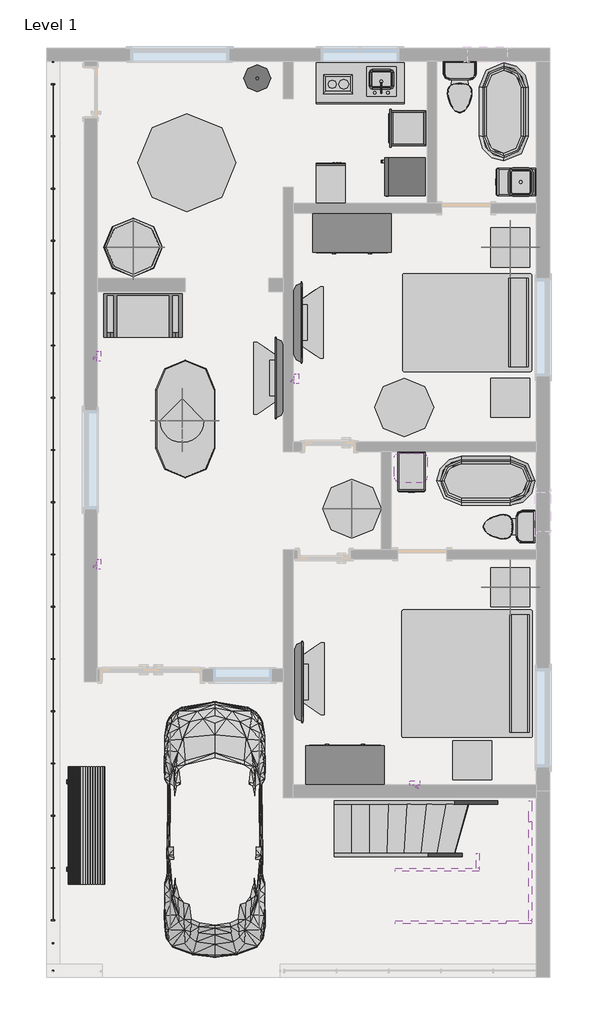
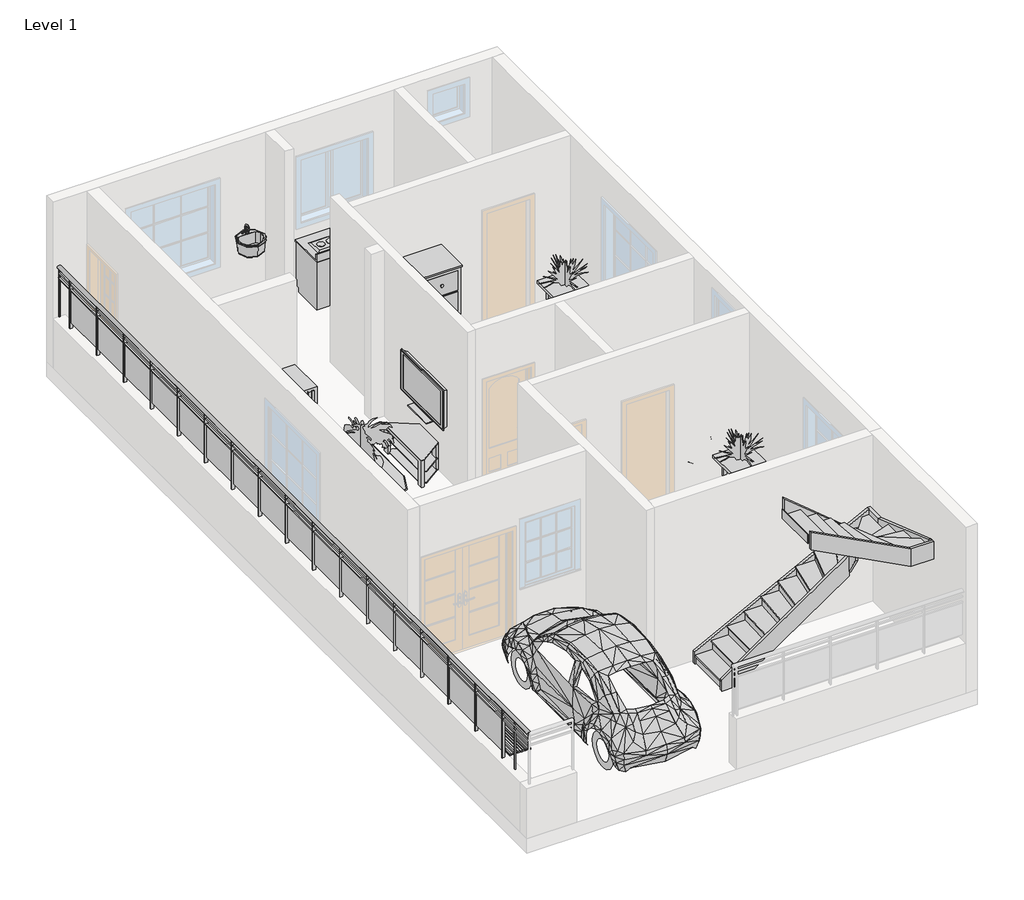
# One storey, part 2 of 2: 23 furniture elements, 10 proxies, 8 flow terminals, 8 members, 6 geographic elements, 1 railing, 1 stair flight.
"""IFC4 building model written with IfcOpenShell, lengths in millimetres."""

from ifc_helpers import new_model, si_unit, point, frame, origin, place, context, project, spatial, polyline, ellipse_curve, trimmed, outline, extrude, transform, mapped, element, save
from ifc_brep_helpers import plane_surface, extruded_surface, advanced_brep
from components import proxy_7e1014cc, proxy_fe84b772, proxy_844211aa, proxy_8b8c2dc4, rpc_beetle_rpc_beetle_3ce7ba48, rpc_picture_frame_rpc_picture_frame_c25e3fe9, proxy_c523a7b7, flow_terminal_871c2e40, flow_terminal_d49f872f, flow_terminal_62a433f7, toilet_domestic_3d_toilet_domestic_3d_f7549cf7, toilet_domestic_3d_toilet_domestic_3d_183bbd19, flow_terminal_b374fae2, furniture_39db8c53, furniture_1fc5af50, furniture_e1791683, furniture_b3f308bd, furniture_9fa109b2, furniture_c333be35, furniture_fdf74506, tv_stand_tv_stand_6ce107e5, furniture_2c34a4f9, furniture_bbcc68ce, furniture_4bee3317, furniture_5bc9ed15, furniture_c80d6d9c, geographic_element_235d1464, rpc_plant_tropical_55f6ff97, rpc_plant_tropical_agave_1_5_93a2a214, rpc_plant_tropical_japanese_fern_2_5_30b4c15b, stair_flight_d882c53c

model = new_model("IFC4")

# Units and contexts
model_context = context("Model", 3, world=origin())
ifc_project = project(units=[si_unit("LENGTHUNIT", "METRE", prefix="MILLI")], contexts=[model_context])

# Site, building, storey
site = spatial("IfcSite", under=ifc_project)
building = spatial("IfcBuilding", under=site)
storey = spatial("IfcBuildingStorey", under=building, Name="Level 1", Elevation=0.0)

# Proxies
placement = place(None, origin())
proxy_shape = proxy_7e1014cc(model_context)
element("IfcBuildingElementProxy", 1, Name="18\" x 24\" x 34 1/2\"", ObjectType="18\" x 24\" x 34 1/2\"", at=placement, inside=storey, context=model_context, shape_type="MappedRepresentation", body=[
    mapped(proxy_shape, transform((-1491.6072765, 12823.4754525, 0.0), x_axis=(-0.9999999999999998, 0.0, 0.0), y_axis=(0.0, -0.9999999999999998, 0.0), z_axis=(0.0, 0.0, 1.0))),
])
proxy_2_shape = proxy_fe84b772(model_context)
element("IfcBuildingElementProxy", 2, Name="Cook Top-2 Unit : 12\" x 18\"", ObjectType="Cook Top-2 Unit : 12\" x 18\"", at=placement, inside=storey, context=model_context, shape_type="MappedRepresentation", body=[
    mapped(proxy_2_shape, transform((-1713.6495405, 14182.6258877, 0.0), x_axis=(0.0, -1.0000000000000004, 0.0), y_axis=(1.0000000000000004, 0.0, 0.0), z_axis=(0.0, 0.0, 1.0))),
])
proxy_3_shape = proxy_844211aa(model_context)
element("IfcBuildingElementProxy", 3, Name="Kitchenette - Small : 54\"", ObjectType="Kitchenette - Small : 54\"", at=placement, inside=storey, context=model_context, shape_type="MappedRepresentation", body=[
    mapped(proxy_3_shape, transform((-1321.78704, 13801.6258877, 0.0), x_axis=(-1.0000000000000004, 0.0, 0.0), y_axis=(0.0, -1.0000000000000004, 0.0), z_axis=(0.0, 0.0, 1.0))),
])
proxy_4_shape = proxy_8b8c2dc4(model_context)
element("IfcBuildingElementProxy", 4, Name="Oven Double-Built-in : 21 1/2\" x 39 1/4\" x 21\"", ObjectType="Oven Double-Built-in : 21 1/2\" x 39 1/4\" x 21\"", at=placement, inside=storey, context=model_context, shape_type="MappedRepresentation", body=[
    mapped(proxy_4_shape, transform((-729.1156039, 13385.4509604, 0.0), x_axis=(0.0, -1.0, 0.0), y_axis=(1.0, 0.0, 0.0), z_axis=(0.0, 0.0, 1.0))),
])
rpc_beetle_rpc_beetle_shape = rpc_beetle_rpc_beetle_3ce7ba48(model_context)
element("IfcBuildingElementProxy", 5, Name="RPC Beetle : RPC Beetle", ObjectType="RPC Beetle : RPC Beetle", at=placement, inside=storey, context=model_context, shape_type="MappedRepresentation", body=[
    mapped(rpc_beetle_rpc_beetle_shape, transform((-3601.1247449, 1279.4258877, 0.0), x_axis=(1.0, 0.0, 0.0), y_axis=(0.0, 1.0, 0.0), z_axis=(0.0, 0.0, 1.0))),
])
rpc_picture_frame_rpc_picture_frame_shape = rpc_picture_frame_rpc_picture_frame_c25e3fe9(model_context)
element("IfcBuildingElementProxy", 6, Name="RPC Picture Frame : RPC Picture Frame", ObjectType="RPC Picture Frame : RPC Picture Frame", at=placement, inside=storey, context=model_context, shape_type="MappedRepresentation", body=[
    mapped(rpc_picture_frame_rpc_picture_frame_shape, transform((-489.6247449, 3209.8258877, 1828.8), x_axis=(-1.0000000000000004, 0.0, 0.0), y_axis=(0.0, -1.0000000000000004, 0.0), z_axis=(0.0, 0.0, 1.0))),
])
element("IfcBuildingElementProxy", 7, Name="RPC Picture Frame : RPC Picture Frame", ObjectType="RPC Picture Frame : RPC Picture Frame", at=placement, inside=storey, context=model_context, shape_type="MappedRepresentation", body=[
    mapped(rpc_picture_frame_rpc_picture_frame_shape, transform((-5429.9247449, 9875.6394183, 1828.8), x_axis=(0.0, 1.0, 0.0), y_axis=(-1.0, 0.0, 0.0), z_axis=(0.0, 0.0, 1.0))),
])
element("IfcBuildingElementProxy", 8, Name="RPC Picture Frame : RPC Picture Frame", ObjectType="RPC Picture Frame : RPC Picture Frame", at=placement, inside=storey, context=model_context, shape_type="MappedRepresentation", body=[
    mapped(rpc_picture_frame_rpc_picture_frame_shape, transform((-5429.9247449, 6639.0450219, 1828.8), x_axis=(0.0, 1.0, 0.0), y_axis=(-1.0, 0.0, 0.0), z_axis=(0.0, 0.0, 1.0))),
])
element("IfcBuildingElementProxy", 9, Name="RPC Picture Frame : RPC Picture Frame", ObjectType="RPC Picture Frame : RPC Picture Frame", at=placement, inside=storey, context=model_context, shape_type="MappedRepresentation", body=[
    mapped(rpc_picture_frame_rpc_picture_frame_shape, transform((-2356.5247449, 9524.6408717, 1828.8), x_axis=(0.0, 1.0, 0.0), y_axis=(-1.0, 0.0, 0.0), z_axis=(0.0, 0.0, 1.0))),
])
proxy_5_shape = proxy_c523a7b7(model_context)
element("IfcBuildingElementProxy", 10, Name="Refrigerator : 24\" x 25\" LH", ObjectType="Refrigerator : 24\" x 25\" LH", at=placement, inside=storey, context=model_context, shape_type="MappedRepresentation", body=[
    mapped(proxy_5_shape, transform((-628.1257735, 12664.9758877, 0.0), x_axis=(0.0, -1.0000000000000007, 0.0), y_axis=(1.0000000000000007, 0.0, 0.0), z_axis=(0.0, 0.0, 1.0))),
])

# Flow terminals
flow_terminal_shape = flow_terminal_871c2e40(model_context)
element("IfcFlowTerminal", 11, ObjectType="Sink Kitchen-Island : 18\" x 18\"", at=placement, inside=storey, context=model_context, shape_type="MappedRepresentation", body=[
    mapped(flow_terminal_shape, transform((-994.6355044, 14146.8712889, 0.0), x_axis=(-1.0000000000000004, 0.0, 0.0), y_axis=(0.0, -1.0000000000000004, 0.0), z_axis=(0.0, 0.0, 1.0))),
])
flow_terminal_2_shape = flow_terminal_d49f872f(model_context)
element("IfcFlowTerminal", 12, ObjectType="Sink Vanity-Round : 19\" x 19\"", at=placement, inside=storey, context=model_context, shape_type="MappedRepresentation", body=[
    mapped(flow_terminal_2_shape, transform((-3037.3764855, 14112.1068919, 609.6), x_axis=(1.0, 0.0, 0.0), y_axis=(0.0, 1.0, 0.0), z_axis=(0.0, 0.0, 1.0))),
])
flow_terminal_3_shape = flow_terminal_62a433f7(model_context)
element("IfcFlowTerminal", 13, ObjectType="Sink Vanity-Square : 20\" x 18\"", at=placement, inside=storey, context=model_context, shape_type="MappedRepresentation", body=[
    mapped(flow_terminal_3_shape, transform((-568.8139855, 8185.8804866, 914.4), x_axis=(1.0, 0.0, 0.0), y_axis=(0.0, 1.0, 0.0), z_axis=(0.0, 0.0, 1.0))),
])
element("IfcFlowTerminal", 14, ObjectType="Sink Vanity-Square : 20\" x 18\"", at=placement, inside=storey, context=model_context, shape_type="MappedRepresentation", body=[
    mapped(flow_terminal_3_shape, transform((1209.8298539, 12598.1151283, 609.6), x_axis=(0.0, -0.9999999999999999, 0.0), y_axis=(0.9999999999999999, 0.0, 0.0), z_axis=(0.0, 0.0, 1.0))),
])
toilet_domestic_3d_toilet_domestic_3d_shape = toilet_domestic_3d_toilet_domestic_3d_f7549cf7(model_context)
toilet_domestic_3d_toilet_domestic_3d_2_shape = toilet_domestic_3d_toilet_domestic_3d_183bbd19(model_context)
element("IfcFlowTerminal", 15, ObjectType="Toilet-Domestic-3D : Toilet-Domestic-3D", at=placement, inside=storey, context=model_context, shape_type="MappedRepresentation", body=[
    mapped(toilet_domestic_3d_toilet_domestic_3d_shape, transform((882.5792277, 7223.0258877, 0.0), x_axis=(0.0, -1.0000000000000004, 0.0), y_axis=(1.0000000000000004, 0.0, 0.0), z_axis=(0.0, 0.0, 1.0))),
    mapped(toilet_domestic_3d_toilet_domestic_3d_2_shape, transform((882.5792277, 7223.0258877, 0.0), x_axis=(0.0, -1.0000000000000004, 0.0), y_axis=(1.0000000000000004, 0.0, 0.0), z_axis=(0.0, 0.0, 1.0))),
])
element("IfcFlowTerminal", 16, ObjectType="Toilet-Domestic-3D : Toilet-Domestic-3D", at=placement, inside=storey, context=model_context, shape_type="MappedRepresentation", body=[
    mapped(toilet_domestic_3d_toilet_domestic_3d_shape, transform((208.8752551, 13967.3298604, 0.0), x_axis=(1.0, 0.0, 0.0), y_axis=(0.0, 1.0, 0.0), z_axis=(0.0, 0.0, 1.0))),
    mapped(toilet_domestic_3d_toilet_domestic_3d_2_shape, transform((208.8752551, 13967.3298604, 0.0), x_axis=(1.0, 0.0, 0.0), y_axis=(0.0, 1.0, 0.0), z_axis=(0.0, 0.0, 1.0))),
])
flow_terminal_4_shape = flow_terminal_b374fae2(model_context)
element("IfcFlowTerminal", 17, ObjectType="Tub-Free Standing-3D : 30\" x 60\"", at=placement, inside=storey, context=model_context, shape_type="MappedRepresentation", body=[
    mapped(flow_terminal_4_shape, transform((894.6752551, 13674.6258877, 0.0), x_axis=(1.0, 0.0, 0.0), y_axis=(0.0, 1.0, 0.0), z_axis=(0.0, 0.0, 1.0))),
])
element("IfcFlowTerminal", 18, ObjectType="Tub-Free Standing-3D : 30\" x 60\"", at=placement, inside=storey, context=model_context, shape_type="MappedRepresentation", body=[
    mapped(flow_terminal_4_shape, transform((615.2752551, 7934.2258877, 0.0), x_axis=(0.0, -1.0000000000000004, 0.0), y_axis=(1.0000000000000004, 0.0, 0.0), z_axis=(0.0, 0.0, 1.0))),
])

# Furniture
furniture_shape = furniture_39db8c53(model_context)
element("IfcFurniture", 19, ObjectType="24\"", at=placement, inside=storey, context=model_context, shape_type="MappedRepresentation", body=[
    mapped(furniture_shape, transform((-559.1624499, 8391.4258877, 0.0), x_axis=(1.0, 0.0, 0.0), y_axis=(0.0, 1.0, 0.0), z_axis=(0.0, 0.0, 1.0))),
])
element("IfcFurniture", 20, ObjectType="24\"", at=placement, inside=storey, context=model_context, shape_type="MappedRepresentation", body=[
    mapped(furniture_shape, transform((1402.6752551, 12601.1635927, 0.0), x_axis=(0.0, -0.9999999999999998, 0.0), y_axis=(0.9999999999999998, 0.0, 0.0), z_axis=(0.0, 0.0, 1.0))),
])
furniture_2_shape = furniture_1fc5af50(model_context)
element("IfcFurniture", 21, ObjectType="Bed-Standard.0001 : King 78\" x 80\"", at=placement, inside=storey, context=model_context, shape_type="MappedRepresentation", body=[
    mapped(furniture_2_shape, transform((368.770337, 5208.5144123, 0.0), x_axis=(0.0, -1.0000000000000002, 0.0), y_axis=(1.0000000000000002, 0.0, 0.0), z_axis=(0.0, 0.0, 1.0))),
])
furniture_3_shape = furniture_e1791683(model_context)
element("IfcFurniture", 22, ObjectType="Bed-Standard.0001 : Queen 60\" x 79\"", at=placement, inside=storey, context=model_context, shape_type="MappedRepresentation", body=[
    mapped(furniture_3_shape, transform((368.770337, 10669.5144123, 0.0), x_axis=(0.0, -1.0000000000000002, 0.0), y_axis=(1.0000000000000002, 0.0, 0.0), z_axis=(0.0, 0.0, 1.0))),
])
furniture_4_shape = furniture_b3f308bd(model_context)
element("IfcFurniture", 23, ObjectType="Counter Top w Sink Hole : 24\" Depth", at=placement, inside=storey, context=model_context, shape_type="MappedRepresentation", body=[
    mapped(furniture_4_shape, transform((-1855.18704, 13801.6258877, 0.0), x_axis=(-1.0000000000000004, 0.0, 0.0), y_axis=(0.0, -1.0000000000000004, 0.0), z_axis=(0.0, 0.0, 1.0))),
])
furniture_5_shape = furniture_9fa109b2(model_context)
element("IfcFurniture", 24, ObjectType="Dresser : 48\" x 72\" x 24\"", at=placement, inside=storey, context=model_context, shape_type="MappedRepresentation", body=[
    mapped(furniture_5_shape, transform((-1845.0542465, 3151.4629336, 0.0), x_axis=(-1.0000000000000004, 0.0, 0.0), y_axis=(0.0, -1.0000000000000004, 0.0), z_axis=(0.0, 0.0, 1.0))),
])
element("IfcFurniture", 25, ObjectType="Dresser : 48\" x 72\" x 24\"", at=placement, inside=storey, context=model_context, shape_type="MappedRepresentation", body=[
    mapped(furniture_5_shape, transform((-1198.3314851, 12158.1888418, 0.0), x_axis=(1.0, 0.0, 0.0), y_axis=(0.0, 1.0, 0.0), z_axis=(0.0, 0.0, 1.0))),
])
furniture_6_shape = furniture_c333be35(model_context)
element("IfcFurniture", 26, ObjectType="Entertainment Center : 72\" x 72\" x 24\"", at=placement, inside=storey, context=model_context, shape_type="MappedRepresentation", body=[
    mapped(furniture_6_shape, transform((-4718.7247449, 10950.4758877, 0.0), x_axis=(1.0, 0.0, 0.0), y_axis=(0.0, 1.0, 0.0), z_axis=(0.0, 0.0, 1.0))),
])
furniture_7_shape = furniture_fdf74506(model_context)
element("IfcFurniture", 27, ObjectType="TV - Flat Screen : 50\"", at=placement, inside=storey, context=model_context, shape_type="MappedRepresentation", body=[
    mapped(furniture_7_shape, transform((-2297.9861213, 4813.9704019, 914.4), x_axis=(0.0, 1.0000000000000002, 0.0), y_axis=(-1.0000000000000002, 0.0, 0.0), z_axis=(0.0, 0.0, 1.0))),
])
element("IfcFurniture", 28, ObjectType="TV - Flat Screen : 50\"", at=placement, inside=storey, context=model_context, shape_type="MappedRepresentation", body=[
    mapped(furniture_7_shape, transform((-2310.6861213, 10401.9704019, 914.4), x_axis=(0.0, 1.0000000000000002, 0.0), y_axis=(-1.0000000000000002, 0.0, 0.0), z_axis=(0.0, 0.0, 1.0))),
])
element("IfcFurniture", 29, ObjectType="TV - Flat Screen : 50\"", at=placement, inside=storey, context=model_context, shape_type="MappedRepresentation", body=[
    mapped(furniture_7_shape, transform((-2592.8633686, 9530.4813736, 914.4), x_axis=(0.0, -1.0000000000000004, 0.0), y_axis=(1.0000000000000004, 0.0, 0.0), z_axis=(0.0, 0.0, 1.0))),
])
tv_stand_tv_stand_shape = tv_stand_tv_stand_6ce107e5(model_context)
element("IfcFurniture", 30, ObjectType="TV Stand : TV Stand", at=placement, inside=storey, context=model_context, shape_type="MappedRepresentation", body=[
    mapped(tv_stand_tv_stand_shape, transform((-2356.5247449, 4735.6378857, 0.0), x_axis=(0.0, 1.0000000000000002, 0.0), y_axis=(-1.0000000000000002, 0.0, 0.0), z_axis=(0.0, 0.0, 1.0))),
])
element("IfcFurniture", 31, ObjectType="TV Stand : TV Stand", at=placement, inside=storey, context=model_context, shape_type="MappedRepresentation", body=[
    mapped(tv_stand_tv_stand_shape, transform((-2369.2247449, 10272.8378857, 0.0), x_axis=(0.0, 1.0000000000000002, 0.0), y_axis=(-1.0000000000000002, 0.0, 0.0), z_axis=(0.0, 0.0, 1.0))),
])
element("IfcFurniture", 32, ObjectType="TV Stand : TV Stand", at=placement, inside=storey, context=model_context, shape_type="MappedRepresentation", body=[
    mapped(tv_stand_tv_stand_shape, transform((-2534.3247449, 9659.6138898, 0.0), x_axis=(0.0, -1.0000000000000004, 0.0), y_axis=(1.0000000000000004, 0.0, 0.0), z_axis=(0.0, 0.0, 1.0))),
])
furniture_8_shape = furniture_2c34a4f9(model_context)
element("IfcFurniture", 33, ObjectType="Table-Dining Oval : 36\" x 72\"", at=placement, inside=storey, context=model_context, shape_type="MappedRepresentation", body=[
    mapped(furniture_8_shape, transform((-4416.4231056, 9301.2455599, 0.0), x_axis=(0.0, 1.0000000000000002, 0.0), y_axis=(-1.0000000000000002, 0.0, 0.0), z_axis=(0.0, 0.0, 1.0))),
])
furniture_9_shape = furniture_bbcc68ce(model_context)
element("IfcFurniture", 34, ObjectType="Table-Dining Round w Chairs : 60\" Diameter", at=placement, inside=storey, context=model_context, shape_type="MappedRepresentation", body=[
    mapped(furniture_9_shape, transform((-4136.6067122, 13072.1045763, 0.0), x_axis=(1.0, 0.0, 0.0), y_axis=(0.0, 1.0, 0.0), z_axis=(0.0, 0.0, 1.0))),
])
furniture_10_shape = furniture_4bee3317(model_context)
element("IfcFurniture", 35, ObjectType="Table-Ellipse : 60\" x 48\"", at=placement, inside=storey, context=model_context, shape_type="MappedRepresentation", body=[
    mapped(furniture_10_shape, transform((-654.7247449, 9077.2258877, 0.0), x_axis=(-1.0000000000000004, 0.0, 0.0), y_axis=(0.0, -1.0000000000000004, 0.0), z_axis=(0.0, 0.0, 1.0))),
])
element("IfcFurniture", 36, ObjectType="Table-Ellipse : 72\" x 36\"", at=placement, inside=storey, context=model_context, shape_type="MappedRepresentation", body=[
    mapped(furniture_10_shape, transform((-1467.5247449, 7502.4258877, 0.0), x_axis=(0.0, 1.0000000000000002, 0.0), y_axis=(-1.0000000000000002, 0.0, 0.0), z_axis=(0.0, 0.0, 1.0))),
])
furniture_11_shape = furniture_5bc9ed15(model_context)
element("IfcFurniture", 37, ObjectType="Table-Night Stand : 24\" x 24\" x 30\"", at=placement, inside=storey, context=model_context, shape_type="MappedRepresentation", body=[
    mapped(furniture_11_shape, transform((687.7416248, 11261.6258877, 0.0), x_axis=(1.0, 0.0, 0.0), y_axis=(0.0, 1.0, 0.0), z_axis=(0.0, 0.0, 1.0))),
])
element("IfcFurniture", 38, ObjectType="Table-Night Stand : 24\" x 24\" x 30\"", at=placement, inside=storey, context=model_context, shape_type="MappedRepresentation", body=[
    mapped(furniture_11_shape, transform((687.7416248, 8924.8258877, 0.0), x_axis=(1.0, 0.0, 0.0), y_axis=(0.0, 1.0, 0.0), z_axis=(0.0, 0.0, 1.0))),
])
element("IfcFurniture", 39, ObjectType="Table-Night Stand : 24\" x 24\" x 30\"", at=placement, inside=storey, context=model_context, shape_type="MappedRepresentation", body=[
    mapped(furniture_11_shape, transform((97.1916248, 3286.0258877, 0.0), x_axis=(1.0, 0.0, 0.0), y_axis=(0.0, 1.0, 0.0), z_axis=(0.0, 0.0, 1.0))),
])
element("IfcFurniture", 40, ObjectType="Table-Night Stand : 24\" x 24\" x 30\"", at=placement, inside=storey, context=model_context, shape_type="MappedRepresentation", body=[
    mapped(furniture_11_shape, transform((687.7416248, 5978.4258877, 0.0), x_axis=(1.0, 0.0, 0.0), y_axis=(0.0, 1.0, 0.0), z_axis=(0.0, 0.0, 1.0))),
])
furniture_12_shape = furniture_c80d6d9c(model_context)
element("IfcFurniture", 41, ObjectType="Table-Round : 36\" Diameter", at=placement, inside=storey, context=model_context, shape_type="MappedRepresentation", body=[
    mapped(furniture_12_shape, transform((-4871.1247449, 11566.4258877, 0.0), x_axis=(1.0, 0.0, 0.0), y_axis=(0.0, 1.0, 0.0), z_axis=(0.0, 0.0, 1.0))),
])

# Geographic elements
geographic_element_shape = geographic_element_235d1464(model_context)
element("IfcGeographicElement", 42, ObjectType="Park Bench : 72\"", at=placement, inside=storey, context=model_context, shape_type="MappedRepresentation", body=[
    mapped(geographic_element_shape, transform((-5633.1247449, 2574.8258877, 0.0), x_axis=(0.0, 1.0, 0.0), y_axis=(-1.0, 0.0, 0.0), z_axis=(0.0, 0.0, 1.0))),
])
rpc_plant_tropical_shape = rpc_plant_tropical_55f6ff97(model_context)
element("IfcGeographicElement", 43, ObjectType="RPC Plant - Tropical", at=placement, inside=storey, context=model_context, shape_type="MappedRepresentation", body=[
    mapped(rpc_plant_tropical_shape, transform((-4871.1247449, 11566.4258877, 762.0), x_axis=(1.0, 0.0, 0.0), y_axis=(0.0, 1.0, 0.0), z_axis=(0.0, 0.0, 1.0))),
])
rpc_plant_tropical_agave_1_5_shape = rpc_plant_tropical_agave_1_5_93a2a214(model_context)
element("IfcGeographicElement", 44, ObjectType="RPC Plant - Tropical : Agave - 1.5'", at=placement, inside=storey, context=model_context, shape_type="MappedRepresentation", body=[
    mapped(rpc_plant_tropical_agave_1_5_shape, transform((-1467.5247449, 7502.4258877, 762.0), x_axis=(1.0, 0.0, 0.0), y_axis=(0.0, 1.0, 0.0), z_axis=(0.0, 0.0, 1.0))),
])
element("IfcGeographicElement", 45, ObjectType="RPC Plant - Tropical : Agave - 1.5'", at=placement, inside=storey, context=model_context, shape_type="MappedRepresentation", body=[
    mapped(rpc_plant_tropical_agave_1_5_shape, transform((996.2752551, 6283.2258877, 762.0), x_axis=(1.0, 0.0, 0.0), y_axis=(0.0, 1.0, 0.0), z_axis=(0.0, 0.0, 1.0))),
])
element("IfcGeographicElement", 46, ObjectType="RPC Plant - Tropical : Agave - 1.5'", at=placement, inside=storey, context=model_context, shape_type="MappedRepresentation", body=[
    mapped(rpc_plant_tropical_agave_1_5_shape, transform((996.2752551, 11566.4258877, 762.0), x_axis=(1.0, 0.0, 0.0), y_axis=(0.0, 1.0, 0.0), z_axis=(0.0, 0.0, 1.0))),
])
rpc_plant_tropical_japanese_fern_2_5_shape = rpc_plant_tropical_japanese_fern_2_5_30b4c15b(model_context)
element("IfcGeographicElement", 47, ObjectType="RPC Plant - Tropical : Japanese Fern - 2.5'", at=placement, inside=storey, context=model_context, shape_type="MappedRepresentation", body=[
    mapped(rpc_plant_tropical_japanese_fern_2_5_shape, transform((-4109.1247449, 8874.0258877, 914.4), x_axis=(1.0, 0.0, 0.0), y_axis=(0.0, 1.0, 0.0), z_axis=(0.0, 0.0, 1.0))),
])

# Members
element("IfcMember", 48, ObjectType="Stringer - 2\" Width", at=placement, inside=storey, context=model_context, shape_type="SweptSolid", body=[
    extrude(outline(polyline([(229.5207224, -1746.1022736), (0.0, -1746.1022736), (0.0, -1526.2011232), (1448.1277826, 1280.536343), (1791.1058444, 1280.536343), (229.5207224, -1746.1022736)])), frame((0.0, 2909.8869757, 0.0), z_axis=(0.0, 1.0, 0.0), x_axis=(0.0, 0.0, 1.0)), (0.0, 0.0, 1.0), 50.8),
])
element("IfcMember", 49, ObjectType="Stringer - 2\" Width", at=placement, inside=storey, context=model_context, shape_type="SweptSolid", body=[
    extrude(outline(polyline([(1280.536343, 2960.6869757), (1331.336343, 2960.6869757), (1331.336343, 2635.3037531), (1280.536343, 2635.3037531), (1280.536343, 2960.6869757)])), frame((0.0, 0.0, 1448.1277826), z_axis=(0.0, 0.0, 1.0), x_axis=(1.0, 0.0, 0.0)), (0.0, 0.0, 1.0), 342.9780618),
])
element("IfcMember", 50, ObjectType="Stringer - 2\" Width", at=placement, inside=storey, context=model_context, shape_type="SweptSolid", body=[
    extrude(outline(polyline([(2635.3037531, 1791.1058444), (2635.3037531, 1448.1277826), (1096.7647998, 1978.265011), (1096.7647998, 2310.1495745), (1128.959821, 2310.1495745), (2635.3037531, 1791.1058444)])), frame((1280.536343, 0.0, 0.0), z_axis=(1.0, 0.0, 0.0), x_axis=(0.0, 1.0, 0.0)), (0.0, 0.0, 1.0), 50.8),
])
element("IfcMember", 51, ObjectType="Stringer - 2\" Width", at=placement, inside=storey, context=model_context, shape_type="SweptSolid", body=[
    extrude(outline(polyline([(1331.336343, 1096.7647998), (1331.336343, 1045.9647998), (930.0452504, 1045.9647998), (930.0452504, 1096.7647998), (1331.336343, 1096.7647998)])), frame((0.0, 0.0, 1987.7625458), z_axis=(0.0, 0.0, 1.0), x_axis=(1.0, 0.0, 0.0)), (0.0, 0.0, 1.0), 322.3870287),
])
element("IfcMember", 52, ObjectType="Stringer - 2\" Width", at=placement, inside=storey, context=model_context, shape_type="SweptSolid", body=[
    extrude(outline(polyline([(197.1288902, -1746.1022736), (0.0, -1746.1022736), (0.0, -1495.0267963), (1349.5812101, 462.8752551), (1719.7763403, 462.8752551), (197.1288902, -1746.1022736)])), frame((0.0, 2092.2258877, 0.0), z_axis=(0.0, 1.0, 0.0), x_axis=(0.0, 0.0, 1.0)), (0.0, 0.0, 1.0), 50.8),
])
element("IfcMember", 53, ObjectType="Stringer - 2\" Width", at=placement, inside=storey, context=model_context, shape_type="SweptSolid", body=[
    extrude(outline(polyline([(2143.0258877, 1935.0678912), (2143.0258877, 1384.5976326), (2126.6177625, 1384.5976326), (1914.4258877, 1725.5306428), (1914.4258877, 2264.7523132), (1937.834975, 2264.7523132), (2143.0258877, 1935.0678912)])), frame((462.8752551, 0.0, 0.0), z_axis=(1.0, 0.0, 0.0), x_axis=(0.0, 1.0, 0.0)), (0.0, 0.0, 1.0), 50.8),
])
element("IfcMember", 54, ObjectType="Stringer - 2\" Width", at=placement, inside=storey, context=model_context, shape_type="SweptSolid", body=[
    extrude(outline(polyline([(1869.9036416, 513.6752551), (2264.7523132, 513.6752551), (3344.3950183, -797.3659919), (2949.5463468, -797.3659919), (1869.9036416, 513.6752551)])), frame((0.0, 1863.6258877, 0.0), z_axis=(0.0, 1.0, 0.0), x_axis=(0.0, 0.0, 1.0)), (0.0, 0.0, 1.0), 50.8),
])
element("IfcMember", 55, ObjectType="Stringer - 2\" Width", at=placement, inside=storey, context=model_context, shape_type="SweptSolid", body=[
    extrude(outline(polyline([(1987.7625458, 930.0452504), (2310.1495745, 930.0452504), (3219.1807534, -797.3659919), (2896.7937247, -797.3659919), (1987.7625458, 930.0452504)])), frame((0.0, 1045.9647998, 0.0), z_axis=(0.0, 1.0, 0.0), x_axis=(0.0, 0.0, 1.0)), (0.0, 0.0, 1.0), 50.8),
])

# Railing
element("IfcRailing", 56, ObjectType="Glass Panel - Bottom Fill", at=placement, inside=storey, context=model_context, shape_type="SolidModel", body=[
    advanced_brep(
    [(-6077.6247449, 14462.0258877, 1828.8), (-6153.8247449, 14462.0258877, 1828.8), (-6077.6247449, 314.2258877, 1828.8), (-6153.8247449, 314.2258877, 1828.8)],
    [
        (0, 1, ellipse_curve(frame((-6115.7247449, 14462.0258877, 1828.8), z_axis=(0.0, 1.0, 0.0), x_axis=(-1.0, 0.0, 0.0)), 38.1, 28.575)),
        (1, 0, ellipse_curve(frame((-6115.7247449, 14462.0258877, 1828.8), z_axis=(0.0, 1.0, 0.0), x_axis=(-1.0, 0.0, 0.0)), 38.1, 28.575)),
        (2, 3, ellipse_curve(frame((-6115.7247449, 314.2258877, 1828.8), z_axis=(0.0, -1.0, 0.0), x_axis=(-1.0, 0.0, 0.0)), 38.1, 28.575)),
        (3, 2, ellipse_curve(frame((-6115.7247449, 314.2258877, 1828.8), z_axis=(0.0, -1.0, 0.0), x_axis=(-1.0, 0.0, 0.0)), 38.1, 28.575)),
        (0, 2),
        (3, 1),
    ],
    [
        plane_surface(frame((-6115.7247449, 14462.0258877, 1828.8), z_axis=(0.0, 1.0, 0.0), x_axis=(0.0, 0.0, -1.0))),
        plane_surface(frame((-6115.7247449, 314.2258877, 1828.8), z_axis=(0.0, -1.0, 0.0), x_axis=(0.0, 0.0, -1.0))),
        extruded_surface(trimmed(ellipse_curve(frame((-6115.7247449, 314.2258877, 1828.8), z_axis=(0.0, 1.0, 0.0), x_axis=(-1.0, 0.0, 0.0)), 38.1, 28.575), [point((-6077.6247449, 314.2258877, 1828.8))], [point((-6153.8247449, 314.2258877, 1828.8))], True, "CARTESIAN"), (0.0, 14147.8, 0.0), 14147.8),
        extruded_surface(trimmed(ellipse_curve(frame((-6115.7247449, 314.2258877, 1828.8), z_axis=(0.0, 1.0, 0.0), x_axis=(-1.0, 0.0, 0.0)), 38.1, 28.575), [point((-6153.8247449, 314.2258877, 1828.8))], [point((-6077.6247449, 314.2258877, 1828.8))], True, "CARTESIAN"), (0.0, 14147.8, 0.0), 14147.8),
    ],
    [
        (0, [[1, 2]]),
        (1, [[3, 4]]),
        (2, [[-1, 5, -4, 6]]),
        (3, [[-2, -6, -3, -5]]),
    ],
),
    extrude(outline(polyline([(-6128.4247449, 14462.0258877), (-6103.0247449, 14462.0258877), (-6103.0247449, 314.2258877), (-6128.4247449, 314.2258877), (-6128.4247449, 14462.0258877)])), frame((0.0, 0.0, 1714.5), z_axis=(0.0, 0.0, 1.0), x_axis=(1.0, 0.0, 0.0)), (0.0, 0.0, 1.0), 25.4),
    extrude(outline(polyline([(-6128.4247449, 14462.0258877), (-6103.0247449, 14462.0258877), (-6103.0247449, 314.2258877), (-6128.4247449, 314.2258877), (-6128.4247449, 14462.0258877)])), frame((0.0, 0.0, 1612.9), z_axis=(0.0, 0.0, 1.0), x_axis=(1.0, 0.0, 0.0)), (0.0, 0.0, 1.0), 25.4),
    extrude(outline(polyline([(-6141.1247449, 1107.9758877), (-6090.3247449, 1107.9758877), (-6090.3247449, 1095.2758877), (-6141.1247449, 1095.2758877), (-6141.1247449, 1107.9758877)])), frame((0.0, 0.0, 914.4), z_axis=(0.0, 0.0, 1.0), x_axis=(1.0, 0.0, 0.0)), (0.0, 0.0, 1.0), 885.6788223),
    extrude(outline(polyline([(-6109.1895879, 1914.4258877), (-6109.1895879, 1101.6258877), (-6115.5395879, 1101.6258877), (-6115.5395879, 1914.4258877), (-6109.1895879, 1914.4258877)])), frame((0.0, 0.0, 1016.0), z_axis=(0.0, 0.0, 1.0), x_axis=(1.0, 0.0, 0.0)), (0.0, 0.0, 1.0), 596.9),
    extrude(outline(polyline([(-6141.1247449, 1920.7758877), (-6090.3247449, 1920.7758877), (-6090.3247449, 1908.0758877), (-6141.1247449, 1908.0758877), (-6141.1247449, 1920.7758877)])), frame((0.0, 0.0, 914.4), z_axis=(0.0, 0.0, 1.0), x_axis=(1.0, 0.0, 0.0)), (0.0, 0.0, 1.0), 885.6788223),
    extrude(outline(polyline([(-6109.1895879, 2727.2258877), (-6109.1895879, 1914.4258877), (-6115.5395879, 1914.4258877), (-6115.5395879, 2727.2258877), (-6109.1895879, 2727.2258877)])), frame((0.0, 0.0, 1016.0), z_axis=(0.0, 0.0, 1.0), x_axis=(1.0, 0.0, 0.0)), (0.0, 0.0, 1.0), 596.9),
    extrude(outline(polyline([(-6141.1247449, 2733.5758877), (-6090.3247449, 2733.5758877), (-6090.3247449, 2720.8758877), (-6141.1247449, 2720.8758877), (-6141.1247449, 2733.5758877)])), frame((0.0, 0.0, 914.4), z_axis=(0.0, 0.0, 1.0), x_axis=(1.0, 0.0, 0.0)), (0.0, 0.0, 1.0), 885.6788223),
    extrude(outline(polyline([(-6109.1895879, 3540.0258877), (-6109.1895879, 2727.2258877), (-6115.5395879, 2727.2258877), (-6115.5395879, 3540.0258877), (-6109.1895879, 3540.0258877)])), frame((0.0, 0.0, 1016.0), z_axis=(0.0, 0.0, 1.0), x_axis=(1.0, 0.0, 0.0)), (0.0, 0.0, 1.0), 596.9),
    extrude(outline(polyline([(-6141.1247449, 3546.3758877), (-6090.3247449, 3546.3758877), (-6090.3247449, 3533.6758877), (-6141.1247449, 3533.6758877), (-6141.1247449, 3546.3758877)])), frame((0.0, 0.0, 914.4), z_axis=(0.0, 0.0, 1.0), x_axis=(1.0, 0.0, 0.0)), (0.0, 0.0, 1.0), 885.6788223),
    extrude(outline(polyline([(-6109.1895879, 4352.8258877), (-6109.1895879, 3540.0258877), (-6115.5395879, 3540.0258877), (-6115.5395879, 4352.8258877), (-6109.1895879, 4352.8258877)])), frame((0.0, 0.0, 1016.0), z_axis=(0.0, 0.0, 1.0), x_axis=(1.0, 0.0, 0.0)), (0.0, 0.0, 1.0), 596.9),
    extrude(outline(polyline([(-6141.1247449, 4359.1758877), (-6090.3247449, 4359.1758877), (-6090.3247449, 4346.4758877), (-6141.1247449, 4346.4758877), (-6141.1247449, 4359.1758877)])), frame((0.0, 0.0, 914.4), z_axis=(0.0, 0.0, 1.0), x_axis=(1.0, 0.0, 0.0)), (0.0, 0.0, 1.0), 885.6788223),
    extrude(outline(polyline([(-6109.1895879, 5165.6258877), (-6109.1895879, 4352.8258877), (-6115.5395879, 4352.8258877), (-6115.5395879, 5165.6258877), (-6109.1895879, 5165.6258877)])), frame((0.0, 0.0, 1016.0), z_axis=(0.0, 0.0, 1.0), x_axis=(1.0, 0.0, 0.0)), (0.0, 0.0, 1.0), 596.9),
    extrude(outline(polyline([(-6141.1247449, 5171.9758877), (-6090.3247449, 5171.9758877), (-6090.3247449, 5159.2758877), (-6141.1247449, 5159.2758877), (-6141.1247449, 5171.9758877)])), frame((0.0, 0.0, 914.4), z_axis=(0.0, 0.0, 1.0), x_axis=(1.0, 0.0, 0.0)), (0.0, 0.0, 1.0), 885.6788223),
    extrude(outline(polyline([(-6109.1895879, 5978.4258877), (-6109.1895879, 5165.6258877), (-6115.5395879, 5165.6258877), (-6115.5395879, 5978.4258877), (-6109.1895879, 5978.4258877)])), frame((0.0, 0.0, 1016.0), z_axis=(0.0, 0.0, 1.0), x_axis=(1.0, 0.0, 0.0)), (0.0, 0.0, 1.0), 596.9),
    extrude(outline(polyline([(-6141.1247449, 5984.7758877), (-6090.3247449, 5984.7758877), (-6090.3247449, 5972.0758877), (-6141.1247449, 5972.0758877), (-6141.1247449, 5984.7758877)])), frame((0.0, 0.0, 914.4), z_axis=(0.0, 0.0, 1.0), x_axis=(1.0, 0.0, 0.0)), (0.0, 0.0, 1.0), 885.6788223),
    extrude(outline(polyline([(-6109.1895879, 6791.2258877), (-6109.1895879, 5978.4258877), (-6115.5395879, 5978.4258877), (-6115.5395879, 6791.2258877), (-6109.1895879, 6791.2258877)])), frame((0.0, 0.0, 1016.0), z_axis=(0.0, 0.0, 1.0), x_axis=(1.0, 0.0, 0.0)), (0.0, 0.0, 1.0), 596.9),
    extrude(outline(polyline([(-6141.1247449, 6797.5758877), (-6090.3247449, 6797.5758877), (-6090.3247449, 6784.8758877), (-6141.1247449, 6784.8758877), (-6141.1247449, 6797.5758877)])), frame((0.0, 0.0, 914.4), z_axis=(0.0, 0.0, 1.0), x_axis=(1.0, 0.0, 0.0)), (0.0, 0.0, 1.0), 885.6788223),
    extrude(outline(polyline([(-6109.1895879, 7604.0258877), (-6109.1895879, 6791.2258877), (-6115.5395879, 6791.2258877), (-6115.5395879, 7604.0258877), (-6109.1895879, 7604.0258877)])), frame((0.0, 0.0, 1016.0), z_axis=(0.0, 0.0, 1.0), x_axis=(1.0, 0.0, 0.0)), (0.0, 0.0, 1.0), 596.9),
    extrude(outline(polyline([(-6141.1247449, 7610.3758877), (-6090.3247449, 7610.3758877), (-6090.3247449, 7597.6758877), (-6141.1247449, 7597.6758877), (-6141.1247449, 7610.3758877)])), frame((0.0, 0.0, 914.4), z_axis=(0.0, 0.0, 1.0), x_axis=(1.0, 0.0, 0.0)), (0.0, 0.0, 1.0), 885.6788223),
    extrude(outline(polyline([(-6109.1895879, 8416.8258877), (-6109.1895879, 7604.0258877), (-6115.5395879, 7604.0258877), (-6115.5395879, 8416.8258877), (-6109.1895879, 8416.8258877)])), frame((0.0, 0.0, 1016.0), z_axis=(0.0, 0.0, 1.0), x_axis=(1.0, 0.0, 0.0)), (0.0, 0.0, 1.0), 596.9),
    extrude(outline(polyline([(-6141.1247449, 8423.1758877), (-6090.3247449, 8423.1758877), (-6090.3247449, 8410.4758877), (-6141.1247449, 8410.4758877), (-6141.1247449, 8423.1758877)])), frame((0.0, 0.0, 914.4), z_axis=(0.0, 0.0, 1.0), x_axis=(1.0, 0.0, 0.0)), (0.0, 0.0, 1.0), 885.6788223),
    extrude(outline(polyline([(-6109.1895879, 9229.6258877), (-6109.1895879, 8416.8258877), (-6115.5395879, 8416.8258877), (-6115.5395879, 9229.6258877), (-6109.1895879, 9229.6258877)])), frame((0.0, 0.0, 1016.0), z_axis=(0.0, 0.0, 1.0), x_axis=(1.0, 0.0, 0.0)), (0.0, 0.0, 1.0), 596.9),
    extrude(outline(polyline([(-6141.1247449, 9235.9758877), (-6090.3247449, 9235.9758877), (-6090.3247449, 9223.2758877), (-6141.1247449, 9223.2758877), (-6141.1247449, 9235.9758877)])), frame((0.0, 0.0, 914.4), z_axis=(0.0, 0.0, 1.0), x_axis=(1.0, 0.0, 0.0)), (0.0, 0.0, 1.0), 885.6788223),
    extrude(outline(polyline([(-6109.1895879, 10042.4258877), (-6109.1895879, 9229.6258877), (-6115.5395879, 9229.6258877), (-6115.5395879, 10042.4258877), (-6109.1895879, 10042.4258877)])), frame((0.0, 0.0, 1016.0), z_axis=(0.0, 0.0, 1.0), x_axis=(1.0, 0.0, 0.0)), (0.0, 0.0, 1.0), 596.9),
    extrude(outline(polyline([(-6141.1247449, 10048.7758877), (-6090.3247449, 10048.7758877), (-6090.3247449, 10036.0758877), (-6141.1247449, 10036.0758877), (-6141.1247449, 10048.7758877)])), frame((0.0, 0.0, 914.4), z_axis=(0.0, 0.0, 1.0), x_axis=(1.0, 0.0, 0.0)), (0.0, 0.0, 1.0), 885.6788223),
    extrude(outline(polyline([(-6109.1895879, 10855.2258877), (-6109.1895879, 10042.4258877), (-6115.5395879, 10042.4258877), (-6115.5395879, 10855.2258877), (-6109.1895879, 10855.2258877)])), frame((0.0, 0.0, 1016.0), z_axis=(0.0, 0.0, 1.0), x_axis=(1.0, 0.0, 0.0)), (0.0, 0.0, 1.0), 596.9),
    extrude(outline(polyline([(-6141.1247449, 10861.5758877), (-6090.3247449, 10861.5758877), (-6090.3247449, 10848.8758877), (-6141.1247449, 10848.8758877), (-6141.1247449, 10861.5758877)])), frame((0.0, 0.0, 914.4), z_axis=(0.0, 0.0, 1.0), x_axis=(1.0, 0.0, 0.0)), (0.0, 0.0, 1.0), 885.6788223),
    extrude(outline(polyline([(-6109.1895879, 11668.0258877), (-6109.1895879, 10855.2258877), (-6115.5395879, 10855.2258877), (-6115.5395879, 11668.0258877), (-6109.1895879, 11668.0258877)])), frame((0.0, 0.0, 1016.0), z_axis=(0.0, 0.0, 1.0), x_axis=(1.0, 0.0, 0.0)), (0.0, 0.0, 1.0), 596.9),
    extrude(outline(polyline([(-6141.1247449, 11674.3758877), (-6090.3247449, 11674.3758877), (-6090.3247449, 11661.6758877), (-6141.1247449, 11661.6758877), (-6141.1247449, 11674.3758877)])), frame((0.0, 0.0, 914.4), z_axis=(0.0, 0.0, 1.0), x_axis=(1.0, 0.0, 0.0)), (0.0, 0.0, 1.0), 885.6788223),
    extrude(outline(polyline([(-6109.1895879, 12480.8258877), (-6109.1895879, 11668.0258877), (-6115.5395879, 11668.0258877), (-6115.5395879, 12480.8258877), (-6109.1895879, 12480.8258877)])), frame((0.0, 0.0, 1016.0), z_axis=(0.0, 0.0, 1.0), x_axis=(1.0, 0.0, 0.0)), (0.0, 0.0, 1.0), 596.9),
    extrude(outline(polyline([(-6141.1247449, 12487.1758877), (-6090.3247449, 12487.1758877), (-6090.3247449, 12474.4758877), (-6141.1247449, 12474.4758877), (-6141.1247449, 12487.1758877)])), frame((0.0, 0.0, 914.4), z_axis=(0.0, 0.0, 1.0), x_axis=(1.0, 0.0, 0.0)), (0.0, 0.0, 1.0), 885.6788223),
    extrude(outline(polyline([(-6109.1895879, 13293.6258877), (-6109.1895879, 12480.8258877), (-6115.5395879, 12480.8258877), (-6115.5395879, 13293.6258877), (-6109.1895879, 13293.6258877)])), frame((0.0, 0.0, 1016.0), z_axis=(0.0, 0.0, 1.0), x_axis=(1.0, 0.0, 0.0)), (0.0, 0.0, 1.0), 596.9),
    extrude(outline(polyline([(-6141.1247449, 13299.9758877), (-6090.3247449, 13299.9758877), (-6090.3247449, 13287.2758877), (-6141.1247449, 13287.2758877), (-6141.1247449, 13299.9758877)])), frame((0.0, 0.0, 914.4), z_axis=(0.0, 0.0, 1.0), x_axis=(1.0, 0.0, 0.0)), (0.0, 0.0, 1.0), 885.6788223),
    extrude(outline(polyline([(-6109.1895879, 14106.4258877), (-6109.1895879, 13293.6258877), (-6115.5395879, 13293.6258877), (-6115.5395879, 14106.4258877), (-6109.1895879, 14106.4258877)])), frame((0.0, 0.0, 1016.0), z_axis=(0.0, 0.0, 1.0), x_axis=(1.0, 0.0, 0.0)), (0.0, 0.0, 1.0), 596.9),
    extrude(outline(polyline([(-6141.1247449, 14112.7758877), (-6090.3247449, 14112.7758877), (-6090.3247449, 14100.0758877), (-6141.1247449, 14100.0758877), (-6141.1247449, 14112.7758877)])), frame((0.0, 0.0, 914.4), z_axis=(0.0, 0.0, 1.0), x_axis=(1.0, 0.0, 0.0)), (0.0, 0.0, 1.0), 885.6788223),
    extrude(outline(polyline([(-6125.2497449, 755.5508877), (-6106.1997449, 755.5508877), (-6106.1997449, 736.5008877), (-6125.2497449, 736.5008877), (-6125.2497449, 755.5508877)])), frame((0.0, 0.0, 914.4), z_axis=(0.0, 0.0, 1.0), x_axis=(1.0, 0.0, 0.0)), (0.0, 0.0, 1.0), 885.6788223),
    extrude(outline(polyline([(-6125.2497449, 326.9258877), (-6106.1997449, 326.9258877), (-6106.1997449, 307.8758877), (-6125.2497449, 307.8758877), (-6125.2497449, 326.9258877)])), frame((0.0, 0.0, 914.4), z_axis=(0.0, 0.0, 1.0), x_axis=(1.0, 0.0, 0.0)), (0.0, 0.0, 1.0), 885.6788223),
    extrude(outline(polyline([(-6125.2497449, 14468.3758877), (-6106.1997449, 14468.3758877), (-6106.1997449, 14449.3258877), (-6125.2497449, 14449.3258877), (-6125.2497449, 14468.3758877)])), frame((0.0, 0.0, 914.4), z_axis=(0.0, 0.0, 1.0), x_axis=(1.0, 0.0, 0.0)), (0.0, 0.0, 1.0), 885.6788223),
])

# Stair flight
stair_flight_shape = stair_flight_d882c53c(model_context)
element("IfcStairFlight", 57, ObjectType="2\" Tread 1\" Nosing 1/4\" Riser", at=placement, inside=storey, context=model_context, shape_type="MappedRepresentation", body=[
    mapped(stair_flight_shape, transform((0.0, 0.0, 0.0), x_axis=(1.0, 0.0, 0.0), y_axis=(0.0, 1.0, 0.0), z_axis=(0.0, 0.0, 1.0))),
])

save(model, "model.ifc")

# Revit data of these elements
# Type "18\" x 24\" x 34 1/2\""
#   Label = "T"
#   Assembly Code = "E1090400"
#   Depth = 2' - 0"
#   Height = 2' - 10 1/2"
#   Width = 1' - 6"
#   Panel Face Material = Plastic, Opaque Black
#   Trach Compact. Material = Steel, Paint Finish, Ivory, Matte
#   Default Elevation = 0
# Type "Cook Top-2 Unit : 12\" x 18\""
#   Assembly Code = "E1090400"
#   Counter Height = 3' - 0"
#   Depth = 1' - 6"
#   Width = 1' - 0"
#   Burner Material = Steel, Chrome Plated
#   Cooktop Material = Steel, Polished
#   Default Elevation = 0
# Type "Kitchenette - Small : 54\""
#   Assembly Code = "E1090400"
#   Width = 4' - 6"
#   Height = 2' - 10 1/2"
#   Depth = 2' - 0"
#   Toe Depth = 0' - 3"
#   Toe Height = 0' - 3 1/2"
#   Cabinet Material = Cabinets
#   Door/Drawer Material = Cabinets
#   Handle Material = Cabinets - Handles
#   Default Elevation = 0
# Type "Oven Double-Built-in : 21 1/2\" x 39 1/4\" x 21\""
#   Label = "OVEN"
#   Assembly Code = "E1090400"
#   Depth = 1' - 9"
#   Height = 3' - 3 1/4"
#   Width = 1' - 9 1/2"
#   Oven Material = Metal - Stainless Steel, Polished
#   Default Elevation = 0
# Type "RPC Beetle : RPC Beetle"
#   built-in parameter 1005195 = "RPC-16-0U6E-L4EG-ENH1-J3KF-SVEL-0TX4-C0"
#   Height = 0
# Type "RPC Picture Frame : RPC Picture Frame"
#   built-in parameter 1005198 = "{2, 15},{39, RPC-16-8M5E-0H3T-F0AH-3U0K-JLQ7-G28B-AU},{1, 0},{1, 0},{2, 19},{1, 8},{5, Color},{1, 0},{1, 0},{3, 0.8},{3, 0.8},{3, 0.8},{1, 8},{7, BBoxMin},{1, 0},{1, 0},{1, 0},{1, 0},{1, 0},{1, 8},{7, BBoxMax},{1, 0},{1, 0},{1, 0},{1, 0},{1, 0},{2, 11},{9, RPCTypeId},{1, 0},{1, 0},{39, RPC-16-8M5E-0H3T-F0AH-3U0K-JLQ7-G28B-AU},{1, 6},{14, RPCPlantHeight},{1, 0},{1, 0},{5, 0.625},{2, 11},{7, keyword},{1, 0},{1, 0},{33, :RPCs:Office Clutter:Geometry:RPC},{2, 11},{8, category},{1, 0},{1, 0},{14, Office Clutter},{2, 11},{12, LocalizedUID},{1, 0},{1, 0},{13, Picture Frame},{2, 14},{6, Height},{1, 0},{1, 0},{5, 0.625},{1, 2},{16, Cast Reflections},{1, 0},{1, 0},{1, 0},{1, 2},{8, Portrait},{1, 0},{1, 0},{1, 1},{1, 2},{5, Stand},{1, 0},{1, 0},{1, 1},{2, 11},{10, RPCL_Frame},{1, 0},{1, 0},{5, Frame},{1, 4},{14, Frame Material},{1, 0},{1, 0},{1, 0},{2, 11},{12, RPCL_Picture},{1, 0},{1, 0},{7, Picture},{2, 11},{15, Picture Preview},{1, 0},{1, 0},{65, __RPC:/object data/textures/object/Photo/Photo0/textures/Portrait},{2, 11},{17, i_Picture Preview},{1, 0},{1, 0},{0, },{1, 2},{18, Use Custom Picture},{1, 0},{1, 0},{1, 0},{2, 11},{17, Picture File Name},{1, 0},{1, 0},{0, },{21, assetlibrary_base.fbx},{1, 5},"
#   built-in parameter 1005195 = "RPC-16-8M5E-0H3T-F0AH-3U0K-JLQ7-G28B-AU"
#   Height = 0
# Type "Refrigerator : 24\" x 25\" LH"
#   Label = "REF."
#   Assembly Code = "E1090400"
#   Depth = 2' - 0 3/4"
#   Handle = 0' - 1 1/2"
#   Height = 5' - 3 1/2"
#   Rear Clearance = 0' - 2"
#   Top Door Height = 1' - 8"
#   Width = 1' - 11 1/2"
#   Material = Steel, Paint Finish, Ivory, Glossy
#   Default Elevation = 0
# Type "Sink Kitchen-Island : 18\" x 18\""
#   Assembly Code = "D2010410"
#   Counter Height = 3' - 0"
#   Depth = 1' - 6"
#   Width = 1' - 6"
#   Faucet Material = Steel, Polished
#   Sink Material = Steel, Polished
#   Default Elevation = 0
# Type "Sink Vanity-Round : 19\" x 19\""
#   Assembly Code = "D2010400"
#   Top Of Counter = 2' - 7"
#   Basin Material = Porcelain, Linen
#   Faucet Material = Steel, Polished
#   Default Elevation = 0
# Type "Sink Vanity-Square : 20\" x 18\""
#   Assembly Code = "D2010400"
#   Counter Height = 2' - 7"
#   Depth = 1' - 6"
#   Width = 1' - 8"
#   Basin Material = Porcelain, Linen
#   Faucet Material = Steel, Polished
#   Default Elevation = 0
# Type "Toilet-Domestic-3D : Toilet-Domestic-3D"
#   Assembly Code = "D2010110"
#   Toilet - Bowl/Basin Material = Porcelain, Linen
#   Toilet - Seat Material = Laminate, Linen, Matte
#   Default Elevation = 0
# Type "Tub-Free Standing-3D : 30\" x 60\""
#   Assembly Code = "D2010110"
#   Height = 1' - 6"
#   Length = 5' - 0"
#   Width = 2' - 6"
#   Tub Material = Porcelain, Ivory
#   Default Elevation = 0
# Type "24\""
#   Assembly Code = "C1030410"
#   Depth = 2' - 0"
#   Height = 2' - 5 1/2"
#   Toe Depth = 0' - 3"
#   Toe Height = 0' - 3 1/2"
#   Width = 1' - 5"
#   Cabinet Material = none
#   Door/Drawer Material = none
#   Handle Material = Cabinets - Handles
#   Default Elevation = 0
# Type "Bed-Standard.0001 : King 78\" x 80\""
#   Assembly Code = "E2020200"
#   Length = 6' - 8"
#   Width = 6' - 6"
#   Leg Material = Steel, Chrome Plated
#   Mattress Material = Linen, Beige
#   Default Elevation = 0
# Type "Bed-Standard.0001 : Queen 60\" x 79\""
#   Assembly Code = "E2020200"
#   Length = 6' - 7"
#   Width = 5' - 0"
#   Leg Material = Steel, Chrome Plated
#   Mattress Material = Linen, White
#   Default Elevation = 0
# Type "Counter Top w Sink Hole : 24\" Depth"
#   Assembly Code = "C1030400"
#   Counter Thickness = 0' - 1 1/2"
#   Depth = 2' - 1"
#   Height = 3' - 0"
#   Length [instance default] = 8' - 0"
#   Sink Location [instance default] = 2' - 0"
#   Sink Location To Wall [instance default] = 0' - 6"
#   Sink Opening Depth [instance default] = 1' - 3"
#   Sink Opening Width [instance default] = 2' - 3"
#   Counter Top Material = none
#   Default Elevation = 0
# Type "Dresser : 48\" x 72\" x 24\""
#   Assembly Code = "E2020200"
#   Depth = 2' - 0"
#   Height = 6' - 0"
#   Width = 4' - 0"
#   Dresser Material = Laminate - Ivory, Glossy
#   Drawer Material = Laminate, Ivory, Matte
#   Knob Material = Cherry
#   Default Elevation = 0
# Type "Entertainment Center : 72\" x 72\" x 24\""
#   Assembly Code = "E2020200"
#   Center Width = 2' - 8"
#   Depth = 2' - 0"
#   Height = 5' - 0"
#   Width = 4' - 0"
#   Material = none
#   Default Elevation = 0
# Type "TV - Flat Screen : 50\""
#   SinAng = 0' - 0.0193"
#   L = 3' - 7.57782"
#   H = 2' - 0.51477"
#   Thickness = 0' - 4.33071"
#   Diagonal = 4' - 2"
#   CosAng = 0' - 0.03431"
#   Stand [instance default] = yes
#   Default Elevation = 0
# Type "TV Stand : TV Stand"
#   Depth = 1' - 6"
#   Width = 3' - 8"
#   Height = 1' - 7 1/2"
#   Finish = Melamine - Gray
#   Default Elevation = 0
# Type "Table-Dining Oval : 36\" x 72\""
#   Assembly Code = "E2020200"
#   Length = 6' - 0"
#   Width = 3' - 0"
#   Base Material = Steel, Chrome Plated
#   Top Material = Glass - Clear, Grey
#   Default Elevation = 0
#   Description = (empty or 0)
# Type "Table-Dining Round w Chairs : 60\" Diameter"
#   Assembly Code = "E2020200"
#   Radius = 2' - 6"
#   Diameter = 5' - 0"
#   Height = 2' - 6"
#   Chairs = 6
#   Base Material = Pine
#   Top Material = Laminate, Linen, Matte
#   Default Elevation = 0
# Type "Table-Ellipse : 60\" x 48\""
#   Assembly Code = "E2020200"
#   Half Width = 1' - 6"
#   Half Length = 1' - 6"
#   Height = 2' - 6"
#   Length = 3' - 0"
#   Width = 3' - 0"
#   Base Material = Birch
#   Top Material = Birch
#   Default Elevation = 0
# Type "Table-Ellipse : 72\" x 36\""
#   Assembly Code = "E2020200"
#   Half Width = 1' - 6"
#   Half Length = 1' - 6"
#   Height = 2' - 6"
#   Length = 3' - 0"
#   Width = 3' - 0"
#   Base Material = Birch
#   Top Material = Laminate - Black
#   Default Elevation = 0
# Type "Table-Night Stand : 24\" x 24\" x 30\""
#   Assembly Code = "E2020200"
#   Depth = 2' - 0"
#   Height = 2' - 6"
#   Width = 2' - 0"
#   Base Material = Birch
#   Top Material = Laminate, Ivory, Matte
#   Default Elevation = 0
# Type "Table-Round : 36\" Diameter"
#   Assembly Code = "E2020200"
#   Base Radius = 0' - 10"
#   Height = 2' - 6"
#   Radius = 1' - 6"
#   Base Material = Steel, Chrome Plated
#   Top Material = Birch
#   Default Elevation = 0
# Type "Park Bench : 72\""
#   Length = 6' - 0"
#   Seat Material = Wood - Teak
#   Frame Material = Steel, Paint Finish, Dark Gray, Matte
# Type "RPC Plant - Tropical"
#   built-in parameter 1005198 = "{2, 15},{39, RPC-16-FWM5-GM7X-C67P-4000-ST1L-LVER-AU},{1, 0},{1, 0},{2, 13},{1, 8},{5, Color},{1, 0},{1, 0},{3, 0.8},{3, 0.8},{3, 0.8},{1, 8},{7, BBoxMin},{1, 0},{1, 0},{1, 0},{1, 0},{1, 0},{1, 8},{7, BBoxMax},{1, 0},{1, 0},{1, 0},{1, 0},{1, 0},{2, 11},{9, RPCTypeId},{1, 0},{1, 0},{39, RPC-16-FWM5-GM7X-C67P-4000-ST1L-LVER-AU},{1, 6},{14, RPCPlantHeight},{1, 0},{1, 0},{1, 3},{2, 11},{7, keyword},{1, 0},{1, 0},{35, :RPCs:Shrubs [General]:Geometry:RPC},{2, 11},{8, category},{1, 0},{1, 0},{16, Shrubs [General]},{2, 11},{12, LocalizedUID},{1, 0},{1, 0},{10, Crane Lily},{2, 14},{6, Height},{1, 0},{1, 0},{1, 3},{1, 2},{16, Cast Reflections},{1, 0},{1, 0},{1, 0},{1, 2},{12, Cast Shadows},{1, 0},{1, 0},{1, 1},{1, 2},{9, Lock View},{1, 0},{1, 0},{1, 0},{1, 4},{5, ViewC},{1, 0},{1, 0},{1, 0},{21, assetlibrary_base.fbx},{1, 5},"
#   built-in parameter 1005195 = "RPC-16-FWM5-GM7X-C67P-4000-ST1L-LVER-AU"
#   Assembly Code = "G2050500"
#   Height = 3' - 0"
#   Default Elevation = 0
# Type "RPC Plant - Tropical : Agave - 1.5'"
#   built-in parameter 1005198 = "{2, 15},{39, RPC-16-G1GJ-63FX-7K5P-N000-ST1L-LVER-AU},{1, 0},{1, 0},{2, 13},{1, 8},{5, Color},{1, 0},{1, 0},{3, 0.8},{3, 0.8},{3, 0.8},{1, 8},{7, BBoxMin},{1, 0},{1, 0},{1, 0},{1, 0},{1, 0},{1, 8},{7, BBoxMax},{1, 0},{1, 0},{1, 0},{1, 0},{1, 0},{2, 11},{9, RPCTypeId},{1, 0},{1, 0},{39, RPC-16-G1GJ-63FX-7K5P-N000-ST1L-LVER-AU},{1, 6},{14, RPCPlantHeight},{1, 0},{1, 0},{3, 1.5},{2, 11},{7, keyword},{1, 0},{1, 0},{35, :RPCs:Plants [General]:Geometry:RPC},{2, 11},{8, category},{1, 0},{1, 0},{16, Plants [General]},{2, 11},{12, LocalizedUID},{1, 0},{1, 0},{5, Agave},{2, 14},{6, Height},{1, 0},{1, 0},{3, 1.5},{1, 2},{16, Cast Reflections},{1, 0},{1, 0},{1, 0},{1, 2},{12, Cast Shadows},{1, 0},{1, 0},{1, 1},{1, 2},{9, Lock View},{1, 0},{1, 0},{1, 0},{1, 4},{5, ViewC},{1, 0},{1, 0},{1, 0},{21, assetlibrary_base.fbx},{1, 5},"
#   built-in parameter 1005195 = "RPC-16-G1GJ-63FX-7K5P-N000-ST1L-LVER-AU"
#   Type Comments = "Agave"
#   Assembly Code = "G2050500"
#   Height = 1' - 6"
#   Default Elevation = 0
# Type "RPC Plant - Tropical : Japanese Fern - 2.5'"
#   built-in parameter 1005198 = "{2, 15},{39, RPC-16-G1GK-JAPX-7J4P-Q000-ST1L-LVER-AU},{1, 0},{1, 0},{2, 13},{1, 8},{5, Color},{1, 0},{1, 0},{3, 0.8},{3, 0.8},{3, 0.8},{1, 8},{7, BBoxMin},{1, 0},{1, 0},{1, 0},{1, 0},{1, 0},{1, 8},{7, BBoxMax},{1, 0},{1, 0},{1, 0},{1, 0},{1, 0},{2, 11},{9, RPCTypeId},{1, 0},{1, 0},{39, RPC-16-G1GK-JAPX-7J4P-Q000-ST1L-LVER-AU},{1, 6},{14, RPCPlantHeight},{1, 0},{1, 0},{3, 2.5},{2, 11},{7, keyword},{1, 0},{1, 0},{35, :RPCs:Shrubs [General]:Geometry:RPC},{2, 11},{8, category},{1, 0},{1, 0},{16, Shrubs [General]},{2, 11},{12, LocalizedUID},{1, 0},{1, 0},{13, Japanese Fern},{2, 14},{6, Height},{1, 0},{1, 0},{3, 2.5},{1, 2},{16, Cast Reflections},{1, 0},{1, 0},{1, 0},{1, 2},{12, Cast Shadows},{1, 0},{1, 0},{1, 1},{1, 2},{9, Lock View},{1, 0},{1, 0},{1, 0},{1, 4},{5, ViewC},{1, 0},{1, 0},{1, 0},{21, assetlibrary_base.fbx},{1, 5},"
#   built-in parameter 1005195 = "RPC-16-G1GK-JAPX-7J4P-Q000-ST1L-LVER-AU"
#   Type Comments = "Japanese Fern"
#   Assembly Code = "G2050500"
#   Height = 2' - 6"
#   Default Elevation = 0
# Type "Glass Panel - Bottom Fill"
#   Assembly Code = "C2010400"
#   built-in parameter 1008612 = 0.0416667 (stored number, unit not read)
#   built-in parameter 1008611 = 0.0416667 (stored number, unit not read)
#   built-in parameter 1008609 = 0.333333 (stored number, unit not read)
#   built-in parameter 1008604 = 0.166667 (stored number, unit not read)
#   built-in parameter 1008603 = 0.166667 (stored number, unit not read)
#   Railing Height = 3' - 0"
#   built-in parameter 1008630 = 2
#   built-in parameter 1008610 = 2
#   built-in parameter 1008618 = Baluster - Square : 3/4"
# Element 1 (IfcBuildingElementProxy, "18\" x 24\" x 34 1/2\"")
#   Phase Created = New Construction
#   Materials on its faces: "Steel, Paint Finish, Ivory, Matte", "Plastic, Opaque Black"
# Element 2 (IfcBuildingElementProxy, "Cook Top-2 Unit : 12\" x 18\"")
#   Phase Created = New Construction
#   Materials on its faces: "Steel, Chrome Plated", "Steel, Polished"
# Element 3 (IfcBuildingElementProxy, "Kitchenette - Small : 54\"")
#   Phase Created = New Construction
#   Materials on its faces: "Cabinets", "Cabinets - Handles"
# Element 4 (IfcBuildingElementProxy, "Oven Double-Built-in : 21 1/2\" x 39 1/4\" x 21\"")
#   Phase Created = New Construction
#   Materials on its faces: "Steel", "Metal - Stainless Steel, Polished", "Glass"
# Element 5 (IfcBuildingElementProxy, "RPC Beetle : RPC Beetle")
#   Phase Created = New Construction
# Elements 6, 7, 8, 9 (IfcBuildingElementProxy, "RPC Picture Frame : RPC Picture Frame")
#   Phase Created = New Construction
# Element 10 (IfcBuildingElementProxy, "Refrigerator : 24\" x 25\" LH")
#   Phase Created = New Construction
#   Materials on its faces: "Steel, Paint Finish, Ivory, Glossy", "Steel, Chrome Plated"
# Element 11 (IfcFlowTerminal, "Sink Kitchen-Island : 18\" x 18\"")
#   Mark = "7"
#   Phase Created = New Construction
#   Materials on its faces: "Steel, Polished"
# Element 12 (IfcFlowTerminal, "Sink Vanity-Round : 19\" x 19\"")
#   Mark = "8"
#   Phase Created = New Construction
#   Materials on its faces: "Porcelain, Linen", "Steel, Polished"
# Element 13 (IfcFlowTerminal, "Sink Vanity-Square : 20\" x 18\"")
#   Mark = "5"
#   Phase Created = New Construction
#   Materials on its faces: "Porcelain, Linen", "Steel, Polished"
# Element 14 (IfcFlowTerminal, "Sink Vanity-Square : 20\" x 18\"")
#   Mark = "6"
#   Phase Created = New Construction
#   Materials on its faces: "Porcelain, Linen", "Steel, Polished"
# Element 15 (IfcFlowTerminal, "Toilet-Domestic-3D : Toilet-Domestic-3D")
#   Mark = "1"
#   Phase Created = New Construction
#   Materials on its faces: "Porcelain, Linen", "Laminate, Linen, Matte"
# Element 16 (IfcFlowTerminal, "Toilet-Domestic-3D : Toilet-Domestic-3D")
#   Mark = "2"
#   Phase Created = New Construction
#   Materials on its faces: "Porcelain, Linen", "Laminate, Linen, Matte"
# Element 17 (IfcFlowTerminal, "Tub-Free Standing-3D : 30\" x 60\"")
#   Mark = "3"
#   Phase Created = New Construction
#   Materials on its faces: "Porcelain, Ivory"
# Element 18 (IfcFlowTerminal, "Tub-Free Standing-3D : 30\" x 60\"")
#   Mark = "4"
#   Phase Created = New Construction
#   Materials on its faces: "Porcelain, Ivory"
# Elements 19, 20 (IfcFurniture, "24\"")
#   Phase Created = New Construction
